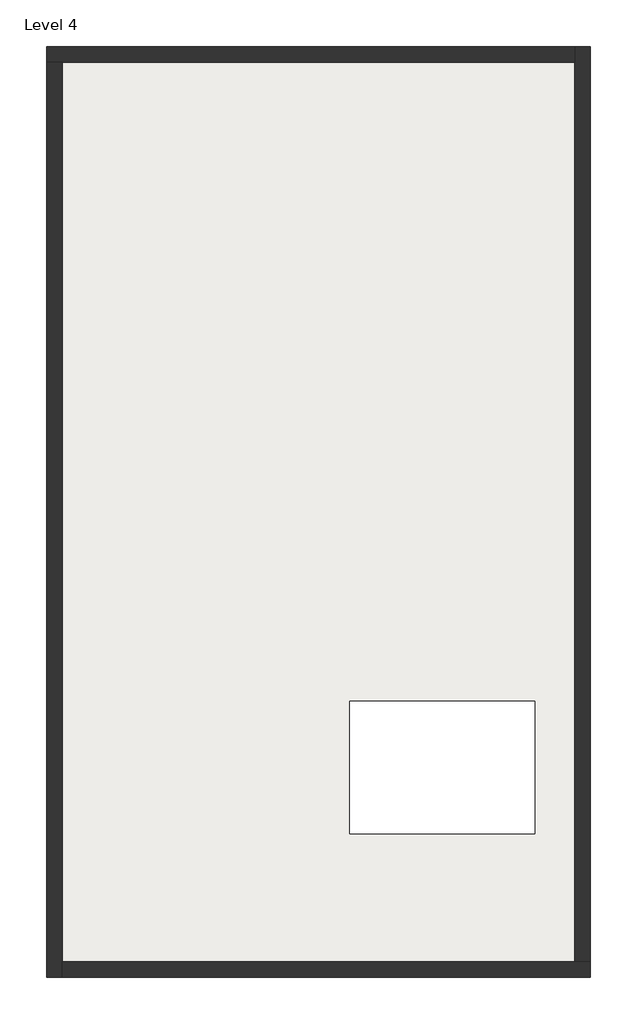
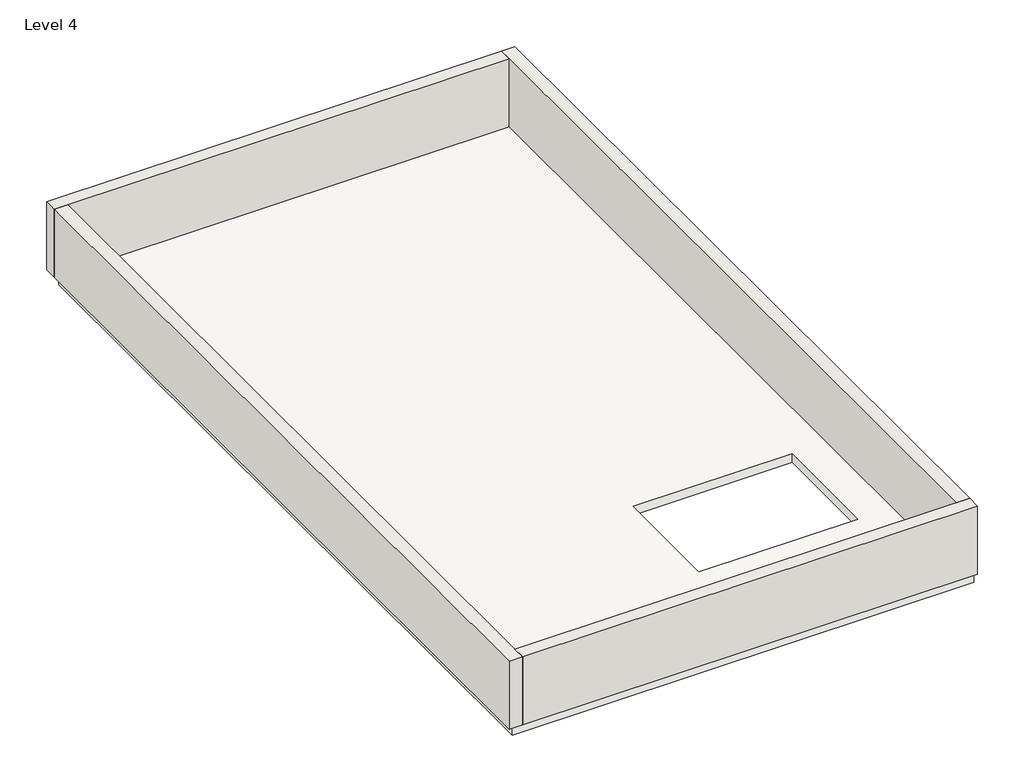
# One storey: 4 walls, 1 roof.
"""IFC4 building model written with IfcOpenShell, lengths in millimetres."""

from ifc_helpers import new_model, si_unit, frame, origin, place, context, project, spatial, polyline, outline, extrude, faceted_brep, element, save

model = new_model("IFC4")

# Units and contexts
model_context = context("Model", 3, world=origin())
ifc_project = project(units=[si_unit("LENGTHUNIT", "METRE", prefix="MILLI")], contexts=[model_context])

# Site, building, storey
site = spatial("IfcSite", under=ifc_project)
building = spatial("IfcBuilding", under=site)
storey = spatial("IfcBuildingStorey", under=building, Name="Level 4", Elevation=6400.8)

# Roof
placement = place(None, origin())
element("IfcRoof", 1, ObjectType="Generic - 12\"", at=placement, inside=storey, context=model_context, shape_type="SweptSolid", body=[
    extrude(outline(polyline([(-5222.940747, -6053.1064015), (-5222.940747, 7243.7935985), (2587.559253, 7243.7935985), (2587.559253, -6053.1064015), (-5222.940747, -6053.1064015)]), holes=[polyline([(1812.859253, -2065.3064015), (-879.540747, -2065.3064015), (-879.540747, -3995.7064015), (1812.859253, -3995.7064015), (1812.859253, -2065.3064015)])]), frame((0.0, 0.0, 6248.4), z_axis=(0.0, 0.0, 1.0), x_axis=(1.0, 0.0, 0.0)), (0.0, 0.0, 1.0), 152.4),
])

# Walls
element("IfcWall", 2, ObjectType="WALL9\"", at=placement, inside=storey, context=model_context, shape_type="Brep", body=[
    faceted_brep([(-5299.140747, 7243.7935985, 6400.8), (-5070.540747, 7243.7935985, 6400.8), (2397.059253, 7243.7935985, 6400.8), (2397.059253, 7243.7935985, 7620.0), (-5070.540747, 7243.7935985, 7620.0), (-5299.140747, 7243.7935985, 7620.0), (-5299.140747, 7472.3935985, 6400.8), (-5299.140747, 7472.3935985, 7620.0), (2397.059253, 7472.3935985, 7620.0), (2397.059253, 7472.3935985, 6400.8)], [[[0, 1, 2, 3, 4, 5]], [[6, 7, 8, 9]], [[2, 1, 0, 6, 9]], [[5, 4, 3, 8, 7]], [[0, 5, 7, 6]], [[3, 2, 9, 8]]]),
])
element("IfcWall", 3, ObjectType="WALL9\"", at=placement, inside=storey, context=model_context, shape_type="Brep", body=[
    faceted_brep([(-5070.540747, -6091.2064015, 6400.8), (-5070.540747, -5862.6064015, 6400.8), (-5070.540747, 7243.7935985, 6400.8), (-5070.540747, 7243.7935985, 7620.0), (-5070.540747, -5862.6064015, 7620.0), (-5070.540747, -6091.2064015, 7620.0), (-5299.140747, -6091.2064015, 6400.8), (-5299.140747, -6091.2064015, 7620.0), (-5299.140747, 7243.7935985, 7620.0), (-5299.140747, 7243.7935985, 6400.8)], [[[0, 1, 2, 3, 4, 5]], [[6, 7, 8, 9]], [[2, 1, 0, 6, 9]], [[5, 4, 3, 8, 7]], [[0, 5, 7, 6]], [[3, 2, 9, 8]]]),
])
element("IfcWall", 4, ObjectType="WALL9\"", at=placement, inside=storey, context=model_context, shape_type="Brep", body=[
    faceted_brep([(2625.659253, -5862.6064015, 6400.8), (2397.059253, -5862.6064015, 6400.8), (-5070.540747, -5862.6064015, 6400.8), (-5070.540747, -5862.6064015, 7620.0), (2397.059253, -5862.6064015, 7620.0), (2625.659253, -5862.6064015, 7620.0), (2625.659253, -6091.2064015, 6400.8), (2625.659253, -6091.2064015, 7620.0), (-5070.540747, -6091.2064015, 7620.0), (-5070.540747, -6091.2064015, 6400.8)], [[[0, 1, 2, 3, 4, 5]], [[6, 7, 8, 9]], [[2, 1, 0, 6, 9]], [[5, 4, 3, 8, 7]], [[0, 5, 7, 6]], [[3, 2, 9, 8]]]),
])
element("IfcWall", 5, ObjectType="WALL9\"", at=placement, inside=storey, context=model_context, shape_type="Brep", body=[
    faceted_brep([(2397.059253, 7472.3935985, 6400.8), (2397.059253, 7243.7935985, 6400.8), (2397.059253, -5862.6064015, 6400.8), (2397.059253, -5862.6064015, 7620.0), (2397.059253, 7243.7935985, 7620.0), (2397.059253, 7472.3935985, 7620.0), (2625.659253, 7472.3935985, 6400.8), (2625.659253, 7472.3935985, 7620.0), (2625.659253, -5862.6064015, 7620.0), (2625.659253, -5862.6064015, 6400.8)], [[[0, 1, 2, 3, 4, 5]], [[6, 7, 8, 9]], [[2, 1, 0, 6, 9]], [[5, 4, 3, 8, 7]], [[0, 5, 7, 6]], [[3, 2, 9, 8]]]),
])

save(model, "model.ifc")

# Revit data of these elements
# Type "Generic - 12\""
#   Assembly Code = "B1020"
#   Layers, outside or top first: 0' - 6" no material (function 1)
# Type "WALL9\""
#   Assembly Code = "B2010"
#   Layers, outside or top first: 0' - 9" no material (function 1)
# Element 1 (IfcRoof, "Generic - 12\"")
#   built-in parameter 1001705 = 21 (stored number, unit not read)
#   built-in parameter 1001701 = -0.5 (stored number, unit not read)
#   built-in parameter 1001710 = 33615
#   Phase Created = New Construction
#   Materials on its faces: "Default Roof"
# Elements 2, 3, 4, 5 (IfcWall, "WALL9\"")
#   Top Offset = 0' - 0"
#   Base Offset = 0' - 0"
#   Unconnected Height = 4' - 0"
#   wall height = 4' - 0"
#   Phase Created = New Construction
#   Base Constraint = Level 4
#   Materials on its faces: "Default Wall", "Blanket"
# Materials
#   "Default Roof": colour RGB 88 101 114, transparency 0, Cost = 0
#   "Default Wall": colour RGB 128 128 128, transparency 0, Cost = 0
#   "Blanket": class "System", colour RGB 59 0 1, transparency 0, Cost = 0
